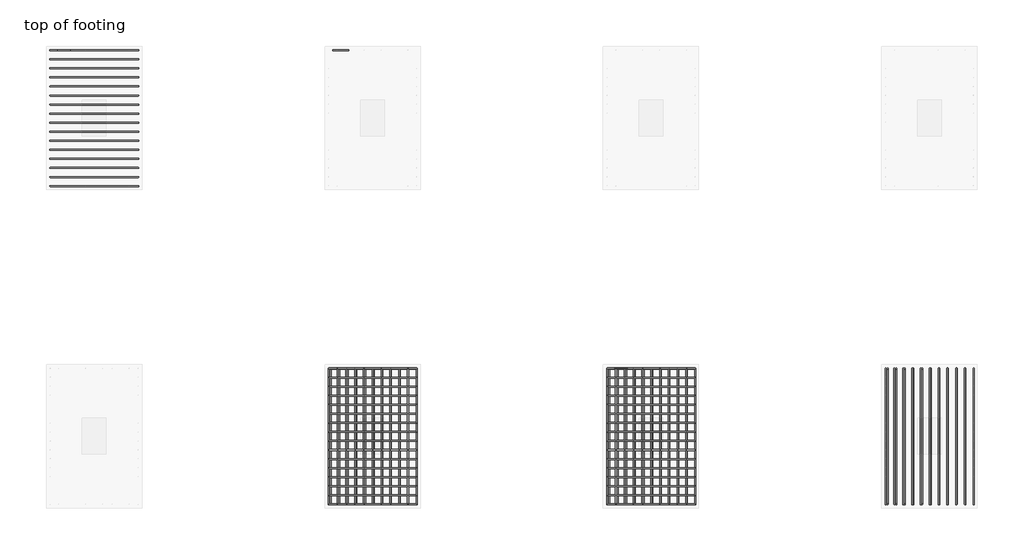
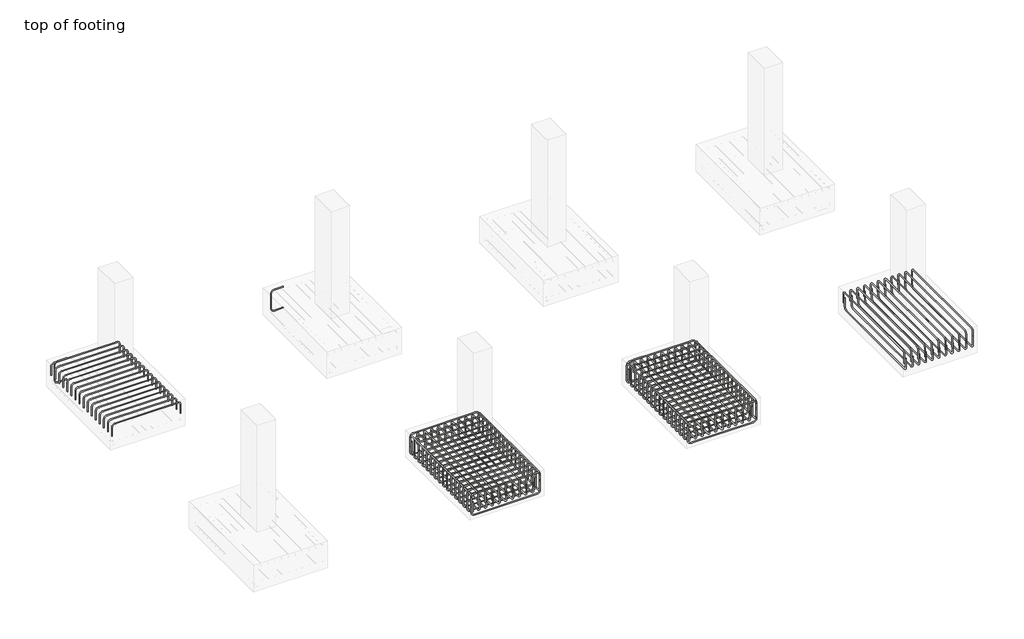
# One storey, part 4 of 8: 14 reinforcing bars.
"""IFC4 building model written with IfcOpenShell, lengths in millimetres."""

from ifc_helpers import new_model, si_unit, point, frame, origin, place, context, project, spatial, polyline, circle_curve, trimmed, segment, composite_curve, source, transform, mapped, element, save
from ifc_brep_helpers import swept_disk

model = new_model("IFC4")

# Units and contexts
model_context = context("Model", 3, world=origin())
ifc_project = project(units=[si_unit("LENGTHUNIT", "METRE", prefix="MILLI")], contexts=[model_context])

# Site, building, storey
site = spatial("IfcSite", under=ifc_project)
building = spatial("IfcBuilding", under=site)
storey = spatial("IfcBuildingStorey", under=building, Name="top of footing", Elevation=-1828.8)

# Reinforcing bars
placement = place(None, origin())
element("IfcReinforcingBar", 1, at=placement, inside=storey, context=model_context, shape_type="SolidModel", body=[
    swept_disk(composite_curve([segment(polyline([(-11543.0309105, 14390.1075251, -2232.45), (-11690.3309105, 14390.1075251, -2232.45)]), True, "CONTINUOUS"), segment(trimmed(circle_curve(frame((-11690.3309105, 14390.1075251, -2186.1), z_axis=(0.0, 1.0, 0.0), x_axis=(0.0, 0.0, -46.34999999999991)), 46.35), [point((-11690.3309105, 14390.1075251, -2232.45))], [point((-11736.6809105, 14390.1075251, -2186.1))], True, "CARTESIAN"), True, "CONTINUOUS"), segment(polyline([(-11736.6809105, 14390.1075251, -2186.1), (-11736.6809105, 14390.1075251, -1921.5)]), True, "CONTINUOUS"), segment(trimmed(circle_curve(frame((-11690.3309105, 14390.1075251, -1921.5), z_axis=(0.0, 1.0, 0.0), x_axis=(-46.349999999998545, 0.0, 0.0)), 46.35), [point((-11736.6809105, 14390.1075251, -1921.5))], [point((-11690.3309105, 14390.1075251, -1875.15))], True, "CARTESIAN"), True, "CONTINUOUS"), segment(polyline([(-11690.3309105, 14390.1075251, -1875.15), (-11543.0309105, 14390.1075251, -1875.15)]), True, "CONTINUOUS")], self_intersect=False), 6.35),
])
reinforcing_bar_shape = source(origin(), model_context, "Body", "SolidModel", [
    swept_disk(composite_curve([segment(polyline([(-11792.7300189, 14390.1075251, -2075.0801535), (-11792.7300189, 14390.1075251, -1927.7801535)]), True, "CONTINUOUS"), segment(trimmed(circle_curve(frame((-11746.3800189, 14390.1075251, -1927.7801535), z_axis=(0.0, 1.0, 0.0), x_axis=(-46.350000000000364, 0.0, 0.0)), 46.35), [point((-11792.7300189, 14390.1075251, -1927.7801535))], [point((-11746.3800189, 14390.1075251, -1881.4301535))], True, "CARTESIAN"), True, "CONTINUOUS"), segment(polyline([(-11746.3800189, 14390.1075251, -1881.4301535), (-10731.7800189, 14390.1075251, -1881.4301535)]), True, "CONTINUOUS"), segment(trimmed(circle_curve(frame((-10731.7800189, 14390.1075251, -1927.7801535), z_axis=(0.0, 1.0, 0.0), x_axis=(0.0, 0.0, 46.350000000000136)), 46.35), [point((-10731.7800189, 14390.1075251, -1881.4301535))], [point((-10685.4300189, 14390.1075251, -1927.7801535))], True, "CARTESIAN"), True, "CONTINUOUS"), segment(polyline([(-10685.4300189, 14390.1075251, -1927.7801535), (-10685.4300189, 14390.1075251, -2075.0801535)]), True, "CONTINUOUS")], self_intersect=False), 6.35),
])
element("IfcReinforcingBar", 2, at=placement, inside=storey, context=model_context, shape_type="MappedRepresentation", body=[
    mapped(reinforcing_bar_shape, transform((0.0, 0.0, 0.0), x_axis=(1.0, 0.0, 0.0), y_axis=(0.0, 1.0, 0.0), z_axis=(0.0, 0.0, 1.0))),
    mapped(reinforcing_bar_shape, transform((0.0, -113.82, 0.0), x_axis=(1.0, 0.0, 0.0), y_axis=(0.0, 1.0, 0.0), z_axis=(0.0, 0.0, 1.0))),
    mapped(reinforcing_bar_shape, transform((0.0, -227.64, 0.0), x_axis=(1.0, 0.0, 0.0), y_axis=(0.0, 1.0, 0.0), z_axis=(0.0, 0.0, 1.0))),
    mapped(reinforcing_bar_shape, transform((0.0, -341.46, 0.0), x_axis=(1.0, 0.0, 0.0), y_axis=(0.0, 1.0, 0.0), z_axis=(0.0, 0.0, 1.0))),
    mapped(reinforcing_bar_shape, transform((0.0, -455.28, 0.0), x_axis=(1.0, 0.0, 0.0), y_axis=(0.0, 1.0, 0.0), z_axis=(0.0, 0.0, 1.0))),
    mapped(reinforcing_bar_shape, transform((0.0, -569.1, 0.0), x_axis=(1.0, 0.0, 0.0), y_axis=(0.0, 1.0, 0.0), z_axis=(0.0, 0.0, 1.0))),
    mapped(reinforcing_bar_shape, transform((0.0, -682.92, 0.0), x_axis=(1.0, 0.0, 0.0), y_axis=(0.0, 1.0, 0.0), z_axis=(0.0, 0.0, 1.0))),
    mapped(reinforcing_bar_shape, transform((0.0, -796.74, 0.0), x_axis=(1.0, 0.0, 0.0), y_axis=(0.0, 1.0, 0.0), z_axis=(0.0, 0.0, 1.0))),
    mapped(reinforcing_bar_shape, transform((0.0, -910.56, 0.0), x_axis=(1.0, 0.0, 0.0), y_axis=(0.0, 1.0, 0.0), z_axis=(0.0, 0.0, 1.0))),
    mapped(reinforcing_bar_shape, transform((0.0, -1024.38, 0.0), x_axis=(1.0, 0.0, 0.0), y_axis=(0.0, 1.0, 0.0), z_axis=(0.0, 0.0, 1.0))),
    mapped(reinforcing_bar_shape, transform((0.0, -1138.2, 0.0), x_axis=(1.0, 0.0, 0.0), y_axis=(0.0, 1.0, 0.0), z_axis=(0.0, 0.0, 1.0))),
    mapped(reinforcing_bar_shape, transform((0.0, -1252.02, 0.0), x_axis=(1.0, 0.0, 0.0), y_axis=(0.0, 1.0, 0.0), z_axis=(0.0, 0.0, 1.0))),
    mapped(reinforcing_bar_shape, transform((0.0, -1365.84, 0.0), x_axis=(1.0, 0.0, 0.0), y_axis=(0.0, 1.0, 0.0), z_axis=(0.0, 0.0, 1.0))),
    mapped(reinforcing_bar_shape, transform((0.0, -1479.66, 0.0), x_axis=(1.0, 0.0, 0.0), y_axis=(0.0, 1.0, 0.0), z_axis=(0.0, 0.0, 1.0))),
    mapped(reinforcing_bar_shape, transform((0.0, -1593.48, 0.0), x_axis=(1.0, 0.0, 0.0), y_axis=(0.0, 1.0, 0.0), z_axis=(0.0, 0.0, 1.0))),
    mapped(reinforcing_bar_shape, transform((0.0, -1707.3, 0.0), x_axis=(1.0, 0.0, 0.0), y_axis=(0.0, 1.0, 0.0), z_axis=(0.0, 0.0, 1.0))),
])
element("IfcReinforcingBar", 3, at=placement, inside=storey, context=model_context, shape_type="SolidModel", body=[
    swept_disk(composite_curve([segment(polyline([(-8043.0309105, 14390.1075251, -2232.45), (-8190.3309105, 14390.1075251, -2232.45)]), True, "CONTINUOUS"), segment(trimmed(circle_curve(frame((-8190.3309105, 14390.1075251, -2186.1), z_axis=(0.0, 1.0, 0.0), x_axis=(0.0, 0.0, -46.34999999999991)), 46.35), [point((-8190.3309105, 14390.1075251, -2232.45))], [point((-8236.6809105, 14390.1075251, -2186.1))], True, "CARTESIAN"), True, "CONTINUOUS"), segment(polyline([(-8236.6809105, 14390.1075251, -2186.1), (-8236.6809105, 14390.1075251, -1921.5)]), True, "CONTINUOUS"), segment(trimmed(circle_curve(frame((-8190.3309105, 14390.1075251, -1921.5), z_axis=(0.0, 1.0, 0.0), x_axis=(-46.349999999999454, 0.0, 0.0)), 46.35), [point((-8236.6809105, 14390.1075251, -1921.5))], [point((-8190.3309105, 14390.1075251, -1875.15))], True, "CARTESIAN"), True, "CONTINUOUS"), segment(polyline([(-8190.3309105, 14390.1075251, -1875.15), (-8043.0309105, 14390.1075251, -1875.15)]), True, "CONTINUOUS")], self_intersect=False), 6.35),
])
reinforcing_bar_2_shape = source(origin(), model_context, "Body", "SolidModel", [
    swept_disk(composite_curve([segment(polyline([(-185.4300189, 8682.8075251, -2014.4920065), (-185.4300189, 8682.8075251, -2161.7920065)]), True, "CONTINUOUS"), segment(trimmed(circle_curve(frame((-185.4300189, 8729.1575251, -2161.7920065), z_axis=(1.0, 0.0, 0.0), x_axis=(0.0, -46.350000000000364, 0.0)), 46.35), [point((-185.4300189, 8682.8075251, -2161.7920065))], [point((-185.4300189, 8729.1575251, -2208.1420065))], True, "CARTESIAN"), True, "CONTINUOUS"), segment(polyline([(-185.4300189, 8729.1575251, -2208.1420065), (-185.4300189, 10343.7575251, -2208.1420065)]), True, "CONTINUOUS"), segment(trimmed(circle_curve(frame((-185.4300189, 10343.7575251, -2161.7920065), z_axis=(1.0, 0.0, 0.0), x_axis=(0.0, 0.0, -46.350000000000364)), 46.35), [point((-185.4300189, 10343.7575251, -2208.1420065))], [point((-185.4300189, 10390.1075251, -2161.7920065))], True, "CARTESIAN"), True, "CONTINUOUS"), segment(polyline([(-185.4300189, 10390.1075251, -2161.7920065), (-185.4300189, 10390.1075251, -2014.4920065)]), True, "CONTINUOUS")], self_intersect=False), 6.35),
])
element("IfcReinforcingBar", 4, at=placement, inside=storey, context=model_context, shape_type="MappedRepresentation", body=[
    mapped(reinforcing_bar_2_shape, transform((0.0, 0.0, 0.0), x_axis=(1.0, 0.0, 0.0), y_axis=(0.0, 1.0, 0.0), z_axis=(0.0, 0.0, 1.0))),
    mapped(reinforcing_bar_2_shape, transform((-108.3645139, 0.0, 0.0), x_axis=(1.0, 0.0, 0.0), y_axis=(0.0, 1.0, 0.0), z_axis=(0.0, 0.0, 1.0))),
    mapped(reinforcing_bar_2_shape, transform((-216.7290279, 0.0, 0.0), x_axis=(1.0, 0.0, 0.0), y_axis=(0.0, 1.0, 0.0), z_axis=(0.0, 0.0, 1.0))),
    mapped(reinforcing_bar_2_shape, transform((-325.0935418, 0.0, 0.0), x_axis=(1.0, 0.0, 0.0), y_axis=(0.0, 1.0, 0.0), z_axis=(0.0, 0.0, 1.0))),
    mapped(reinforcing_bar_2_shape, transform((-433.4580557, 0.0, 0.0), x_axis=(1.0, 0.0, 0.0), y_axis=(0.0, 1.0, 0.0), z_axis=(0.0, 0.0, 1.0))),
    mapped(reinforcing_bar_2_shape, transform((-541.8225696, 0.0, 0.0), x_axis=(1.0, 0.0, 0.0), y_axis=(0.0, 1.0, 0.0), z_axis=(0.0, 0.0, 1.0))),
    mapped(reinforcing_bar_2_shape, transform((-650.1870836, 0.0, 0.0), x_axis=(1.0, 0.0, 0.0), y_axis=(0.0, 1.0, 0.0), z_axis=(0.0, 0.0, 1.0))),
    mapped(reinforcing_bar_2_shape, transform((-758.5515975, 0.0, 0.0), x_axis=(1.0, 0.0, 0.0), y_axis=(0.0, 1.0, 0.0), z_axis=(0.0, 0.0, 1.0))),
    mapped(reinforcing_bar_2_shape, transform((-866.9161114, 0.0, 0.0), x_axis=(1.0, 0.0, 0.0), y_axis=(0.0, 1.0, 0.0), z_axis=(0.0, 0.0, 1.0))),
    mapped(reinforcing_bar_2_shape, transform((-975.2806253, 0.0, 0.0), x_axis=(1.0, 0.0, 0.0), y_axis=(0.0, 1.0, 0.0), z_axis=(0.0, 0.0, 1.0))),
    mapped(reinforcing_bar_2_shape, transform((-1083.6451393, 0.0, 0.0), x_axis=(1.0, 0.0, 0.0), y_axis=(0.0, 1.0, 0.0), z_axis=(0.0, 0.0, 1.0))),
])
reinforcing_bar_3_shape = source(origin(), model_context, "Body", "SolidModel", [
    swept_disk(composite_curve([segment(polyline([(-1292.7300189, 8682.8075251, -2085.8010212), (-1292.7300189, 8682.8075251, -1938.5010212)]), True, "CONTINUOUS"), segment(trimmed(circle_curve(frame((-1292.7300189, 8729.1575251, -1938.5010212), z_axis=(-1.0, 0.0, 0.0), x_axis=(0.0, -46.350000000000364, 0.0)), 46.35), [point((-1292.7300189, 8682.8075251, -1938.5010212))], [point((-1292.7300189, 8729.1575251, -1892.1510212))], True, "CARTESIAN"), True, "CONTINUOUS"), segment(polyline([(-1292.7300189, 8729.1575251, -1892.1510212), (-1292.7300189, 10343.7575251, -1892.1510212)]), True, "CONTINUOUS"), segment(trimmed(circle_curve(frame((-1292.7300189, 10343.7575251, -1938.5010212), z_axis=(-1.0, 0.0, 0.0), x_axis=(0.0, 0.0, 46.34999999999991)), 46.35), [point((-1292.7300189, 10343.7575251, -1892.1510212))], [point((-1292.7300189, 10390.1075251, -1938.5010212))], True, "CARTESIAN"), True, "CONTINUOUS"), segment(polyline([(-1292.7300189, 10390.1075251, -1938.5010212), (-1292.7300189, 10390.1075251, -2085.8010212)]), True, "CONTINUOUS")], self_intersect=False), 6.35),
])
element("IfcReinforcingBar", 5, at=placement, inside=storey, context=model_context, shape_type="MappedRepresentation", body=[
    mapped(reinforcing_bar_3_shape, transform((0.0, 0.0, 0.0), x_axis=(1.0, 0.0, 0.0), y_axis=(0.0, 1.0, 0.0), z_axis=(0.0, 0.0, 1.0))),
    mapped(reinforcing_bar_3_shape, transform((110.73, 0.0, 0.0), x_axis=(1.0, 0.0, 0.0), y_axis=(0.0, 1.0, 0.0), z_axis=(0.0, 0.0, 1.0))),
    mapped(reinforcing_bar_3_shape, transform((221.46, 0.0, 0.0), x_axis=(1.0, 0.0, 0.0), y_axis=(0.0, 1.0, 0.0), z_axis=(0.0, 0.0, 1.0))),
    mapped(reinforcing_bar_3_shape, transform((332.19, 0.0, 0.0), x_axis=(1.0, 0.0, 0.0), y_axis=(0.0, 1.0, 0.0), z_axis=(0.0, 0.0, 1.0))),
    mapped(reinforcing_bar_3_shape, transform((442.92, 0.0, 0.0), x_axis=(1.0, 0.0, 0.0), y_axis=(0.0, 1.0, 0.0), z_axis=(0.0, 0.0, 1.0))),
    mapped(reinforcing_bar_3_shape, transform((553.65, 0.0, 0.0), x_axis=(1.0, 0.0, 0.0), y_axis=(0.0, 1.0, 0.0), z_axis=(0.0, 0.0, 1.0))),
    mapped(reinforcing_bar_3_shape, transform((664.38, 0.0, 0.0), x_axis=(1.0, 0.0, 0.0), y_axis=(0.0, 1.0, 0.0), z_axis=(0.0, 0.0, 1.0))),
    mapped(reinforcing_bar_3_shape, transform((775.11, 0.0, 0.0), x_axis=(1.0, 0.0, 0.0), y_axis=(0.0, 1.0, 0.0), z_axis=(0.0, 0.0, 1.0))),
    mapped(reinforcing_bar_3_shape, transform((885.84, 0.0, 0.0), x_axis=(1.0, 0.0, 0.0), y_axis=(0.0, 1.0, 0.0), z_axis=(0.0, 0.0, 1.0))),
    mapped(reinforcing_bar_3_shape, transform((996.57, 0.0, 0.0), x_axis=(1.0, 0.0, 0.0), y_axis=(0.0, 1.0, 0.0), z_axis=(0.0, 0.0, 1.0))),
    mapped(reinforcing_bar_3_shape, transform((1107.3, 0.0, 0.0), x_axis=(1.0, 0.0, 0.0), y_axis=(0.0, 1.0, 0.0), z_axis=(0.0, 0.0, 1.0))),
])
reinforcing_bar_4_shape = source(origin(), model_context, "Body", "SolidModel", [
    swept_disk(composite_curve([segment(polyline([(-3685.4300189, 8682.8075251, -2014.4920065), (-3685.4300189, 8682.8075251, -2161.7920065)]), True, "CONTINUOUS"), segment(trimmed(circle_curve(frame((-3685.4300189, 8729.1575251, -2161.7920065), z_axis=(1.0, 0.0, 0.0), x_axis=(0.0, -46.350000000000364, 0.0)), 46.35), [point((-3685.4300189, 8682.8075251, -2161.7920065))], [point((-3685.4300189, 8729.1575251, -2208.1420065))], True, "CARTESIAN"), True, "CONTINUOUS"), segment(polyline([(-3685.4300189, 8729.1575251, -2208.1420065), (-3685.4300189, 10343.7575251, -2208.1420065)]), True, "CONTINUOUS"), segment(trimmed(circle_curve(frame((-3685.4300189, 10343.7575251, -2161.7920065), z_axis=(1.0, 0.0, 0.0), x_axis=(0.0, 0.0, -46.350000000000364)), 46.35), [point((-3685.4300189, 10343.7575251, -2208.1420065))], [point((-3685.4300189, 10390.1075251, -2161.7920065))], True, "CARTESIAN"), True, "CONTINUOUS"), segment(polyline([(-3685.4300189, 10390.1075251, -2161.7920065), (-3685.4300189, 10390.1075251, -2014.4920065)]), True, "CONTINUOUS")], self_intersect=False), 6.35),
])
element("IfcReinforcingBar", 6, at=placement, inside=storey, context=model_context, shape_type="MappedRepresentation", body=[
    mapped(reinforcing_bar_4_shape, transform((0.0, 0.0, 0.0), x_axis=(1.0, 0.0, 0.0), y_axis=(0.0, 1.0, 0.0), z_axis=(0.0, 0.0, 1.0))),
    mapped(reinforcing_bar_4_shape, transform((-108.3645139, 0.0, 0.0), x_axis=(1.0, 0.0, 0.0), y_axis=(0.0, 1.0, 0.0), z_axis=(0.0, 0.0, 1.0))),
    mapped(reinforcing_bar_4_shape, transform((-216.7290279, 0.0, 0.0), x_axis=(1.0, 0.0, 0.0), y_axis=(0.0, 1.0, 0.0), z_axis=(0.0, 0.0, 1.0))),
    mapped(reinforcing_bar_4_shape, transform((-325.0935418, 0.0, 0.0), x_axis=(1.0, 0.0, 0.0), y_axis=(0.0, 1.0, 0.0), z_axis=(0.0, 0.0, 1.0))),
    mapped(reinforcing_bar_4_shape, transform((-433.4580557, 0.0, 0.0), x_axis=(1.0, 0.0, 0.0), y_axis=(0.0, 1.0, 0.0), z_axis=(0.0, 0.0, 1.0))),
    mapped(reinforcing_bar_4_shape, transform((-541.8225696, 0.0, 0.0), x_axis=(1.0, 0.0, 0.0), y_axis=(0.0, 1.0, 0.0), z_axis=(0.0, 0.0, 1.0))),
    mapped(reinforcing_bar_4_shape, transform((-650.1870836, 0.0, 0.0), x_axis=(1.0, 0.0, 0.0), y_axis=(0.0, 1.0, 0.0), z_axis=(0.0, 0.0, 1.0))),
    mapped(reinforcing_bar_4_shape, transform((-758.5515975, 0.0, 0.0), x_axis=(1.0, 0.0, 0.0), y_axis=(0.0, 1.0, 0.0), z_axis=(0.0, 0.0, 1.0))),
    mapped(reinforcing_bar_4_shape, transform((-866.9161114, 0.0, 0.0), x_axis=(1.0, 0.0, 0.0), y_axis=(0.0, 1.0, 0.0), z_axis=(0.0, 0.0, 1.0))),
    mapped(reinforcing_bar_4_shape, transform((-975.2806253, 0.0, 0.0), x_axis=(1.0, 0.0, 0.0), y_axis=(0.0, 1.0, 0.0), z_axis=(0.0, 0.0, 1.0))),
    mapped(reinforcing_bar_4_shape, transform((-1083.6451393, 0.0, 0.0), x_axis=(1.0, 0.0, 0.0), y_axis=(0.0, 1.0, 0.0), z_axis=(0.0, 0.0, 1.0))),
])
reinforcing_bar_5_shape = source(origin(), model_context, "Body", "SolidModel", [
    swept_disk(composite_curve([segment(polyline([(-4792.7300189, 8682.8075251, -2085.8010212), (-4792.7300189, 8682.8075251, -1938.5010212)]), True, "CONTINUOUS"), segment(trimmed(circle_curve(frame((-4792.7300189, 8729.1575251, -1938.5010212), z_axis=(-1.0, 0.0, 0.0), x_axis=(0.0, -46.350000000000364, 0.0)), 46.35), [point((-4792.7300189, 8682.8075251, -1938.5010212))], [point((-4792.7300189, 8729.1575251, -1892.1510212))], True, "CARTESIAN"), True, "CONTINUOUS"), segment(polyline([(-4792.7300189, 8729.1575251, -1892.1510212), (-4792.7300189, 10343.7575251, -1892.1510212)]), True, "CONTINUOUS"), segment(trimmed(circle_curve(frame((-4792.7300189, 10343.7575251, -1938.5010212), z_axis=(-1.0, 0.0, 0.0), x_axis=(0.0, 0.0, 46.34999999999991)), 46.35), [point((-4792.7300189, 10343.7575251, -1892.1510212))], [point((-4792.7300189, 10390.1075251, -1938.5010212))], True, "CARTESIAN"), True, "CONTINUOUS"), segment(polyline([(-4792.7300189, 10390.1075251, -1938.5010212), (-4792.7300189, 10390.1075251, -2085.8010212)]), True, "CONTINUOUS")], self_intersect=False), 6.35),
])
element("IfcReinforcingBar", 7, at=placement, inside=storey, context=model_context, shape_type="MappedRepresentation", body=[
    mapped(reinforcing_bar_5_shape, transform((0.0, 0.0, 0.0), x_axis=(1.0, 0.0, 0.0), y_axis=(0.0, 1.0, 0.0), z_axis=(0.0, 0.0, 1.0))),
    mapped(reinforcing_bar_5_shape, transform((110.73, 0.0, 0.0), x_axis=(1.0, 0.0, 0.0), y_axis=(0.0, 1.0, 0.0), z_axis=(0.0, 0.0, 1.0))),
    mapped(reinforcing_bar_5_shape, transform((221.46, 0.0, 0.0), x_axis=(1.0, 0.0, 0.0), y_axis=(0.0, 1.0, 0.0), z_axis=(0.0, 0.0, 1.0))),
    mapped(reinforcing_bar_5_shape, transform((332.19, 0.0, 0.0), x_axis=(1.0, 0.0, 0.0), y_axis=(0.0, 1.0, 0.0), z_axis=(0.0, 0.0, 1.0))),
    mapped(reinforcing_bar_5_shape, transform((442.92, 0.0, 0.0), x_axis=(1.0, 0.0, 0.0), y_axis=(0.0, 1.0, 0.0), z_axis=(0.0, 0.0, 1.0))),
    mapped(reinforcing_bar_5_shape, transform((553.65, 0.0, 0.0), x_axis=(1.0, 0.0, 0.0), y_axis=(0.0, 1.0, 0.0), z_axis=(0.0, 0.0, 1.0))),
    mapped(reinforcing_bar_5_shape, transform((664.38, 0.0, 0.0), x_axis=(1.0, 0.0, 0.0), y_axis=(0.0, 1.0, 0.0), z_axis=(0.0, 0.0, 1.0))),
    mapped(reinforcing_bar_5_shape, transform((775.11, 0.0, 0.0), x_axis=(1.0, 0.0, 0.0), y_axis=(0.0, 1.0, 0.0), z_axis=(0.0, 0.0, 1.0))),
    mapped(reinforcing_bar_5_shape, transform((885.84, 0.0, 0.0), x_axis=(1.0, 0.0, 0.0), y_axis=(0.0, 1.0, 0.0), z_axis=(0.0, 0.0, 1.0))),
    mapped(reinforcing_bar_5_shape, transform((996.57, 0.0, 0.0), x_axis=(1.0, 0.0, 0.0), y_axis=(0.0, 1.0, 0.0), z_axis=(0.0, 0.0, 1.0))),
    mapped(reinforcing_bar_5_shape, transform((1107.3, 0.0, 0.0), x_axis=(1.0, 0.0, 0.0), y_axis=(0.0, 1.0, 0.0), z_axis=(0.0, 0.0, 1.0))),
])
element("IfcReinforcingBar", 8, at=placement, inside=storey, context=model_context, shape_type="SolidModel", body=[
    swept_disk(composite_curve([segment(polyline([(-4543.0309105, 10390.1075251, -2232.45), (-4690.3309105, 10390.1075251, -2232.45)]), True, "CONTINUOUS"), segment(trimmed(circle_curve(frame((-4690.3309105, 10390.1075251, -2186.1), z_axis=(0.0, 1.0, 0.0), x_axis=(0.0, 0.0, -46.34999999999991)), 46.35), [point((-4690.3309105, 10390.1075251, -2232.45))], [point((-4736.6809105, 10390.1075251, -2186.1))], True, "CARTESIAN"), True, "CONTINUOUS"), segment(polyline([(-4736.6809105, 10390.1075251, -2186.1), (-4736.6809105, 10390.1075251, -1921.5)]), True, "CONTINUOUS"), segment(trimmed(circle_curve(frame((-4690.3309105, 10390.1075251, -1921.5), z_axis=(0.0, 1.0, 0.0), x_axis=(-46.350000000000364, 0.0, 0.0)), 46.35), [point((-4736.6809105, 10390.1075251, -1921.5))], [point((-4690.3309105, 10390.1075251, -1875.15))], True, "CARTESIAN"), True, "CONTINUOUS"), segment(polyline([(-4690.3309105, 10390.1075251, -1875.15), (-4543.0309105, 10390.1075251, -1875.15)]), True, "CONTINUOUS")], self_intersect=False), 6.35),
])
reinforcing_bar_6_shape = source(origin(), model_context, "Body", "SolidModel", [
    swept_disk(composite_curve([segment(polyline([(-3685.4300189, 10390.1075251, -2044.8290141), (-3685.4300189, 10390.1075251, -2192.1290141)]), True, "CONTINUOUS"), segment(trimmed(circle_curve(frame((-3731.7800189, 10390.1075251, -2192.1290141), z_axis=(0.0, 1.0, 0.0), x_axis=(46.34999999999991, 0.0, 0.0)), 46.35), [point((-3685.4300189, 10390.1075251, -2192.1290141))], [point((-3731.7800189, 10390.1075251, -2238.4790141))], True, "CARTESIAN"), True, "CONTINUOUS"), segment(polyline([(-3731.7800189, 10390.1075251, -2238.4790141), (-4746.3800189, 10390.1075251, -2238.4790141)]), True, "CONTINUOUS"), segment(trimmed(circle_curve(frame((-4746.3800189, 10390.1075251, -2192.1290141), z_axis=(0.0, 1.0, 0.0), x_axis=(0.0, 0.0, -46.34999999999991)), 46.35), [point((-4746.3800189, 10390.1075251, -2238.4790141))], [point((-4792.7300189, 10390.1075251, -2192.1290141))], True, "CARTESIAN"), True, "CONTINUOUS"), segment(polyline([(-4792.7300189, 10390.1075251, -2192.1290141), (-4792.7300189, 10390.1075251, -2044.8290141)]), True, "CONTINUOUS")], self_intersect=False), 6.35),
])
element("IfcReinforcingBar", 9, at=placement, inside=storey, context=model_context, shape_type="MappedRepresentation", body=[
    mapped(reinforcing_bar_6_shape, transform((0.0, 0.0, 0.0), x_axis=(1.0, 0.0, 0.0), y_axis=(0.0, 1.0, 0.0), z_axis=(0.0, 0.0, 1.0))),
    mapped(reinforcing_bar_6_shape, transform((0.0, -113.82, 0.0), x_axis=(1.0, 0.0, 0.0), y_axis=(0.0, 1.0, 0.0), z_axis=(0.0, 0.0, 1.0))),
    mapped(reinforcing_bar_6_shape, transform((0.0, -227.64, 0.0), x_axis=(1.0, 0.0, 0.0), y_axis=(0.0, 1.0, 0.0), z_axis=(0.0, 0.0, 1.0))),
    mapped(reinforcing_bar_6_shape, transform((0.0, -341.46, 0.0), x_axis=(1.0, 0.0, 0.0), y_axis=(0.0, 1.0, 0.0), z_axis=(0.0, 0.0, 1.0))),
    mapped(reinforcing_bar_6_shape, transform((0.0, -455.28, 0.0), x_axis=(1.0, 0.0, 0.0), y_axis=(0.0, 1.0, 0.0), z_axis=(0.0, 0.0, 1.0))),
    mapped(reinforcing_bar_6_shape, transform((0.0, -569.1, 0.0), x_axis=(1.0, 0.0, 0.0), y_axis=(0.0, 1.0, 0.0), z_axis=(0.0, 0.0, 1.0))),
    mapped(reinforcing_bar_6_shape, transform((0.0, -682.92, 0.0), x_axis=(1.0, 0.0, 0.0), y_axis=(0.0, 1.0, 0.0), z_axis=(0.0, 0.0, 1.0))),
    mapped(reinforcing_bar_6_shape, transform((0.0, -796.74, 0.0), x_axis=(1.0, 0.0, 0.0), y_axis=(0.0, 1.0, 0.0), z_axis=(0.0, 0.0, 1.0))),
    mapped(reinforcing_bar_6_shape, transform((0.0, -910.56, 0.0), x_axis=(1.0, 0.0, 0.0), y_axis=(0.0, 1.0, 0.0), z_axis=(0.0, 0.0, 1.0))),
    mapped(reinforcing_bar_6_shape, transform((0.0, -1024.38, 0.0), x_axis=(1.0, 0.0, 0.0), y_axis=(0.0, 1.0, 0.0), z_axis=(0.0, 0.0, 1.0))),
    mapped(reinforcing_bar_6_shape, transform((0.0, -1138.2, 0.0), x_axis=(1.0, 0.0, 0.0), y_axis=(0.0, 1.0, 0.0), z_axis=(0.0, 0.0, 1.0))),
    mapped(reinforcing_bar_6_shape, transform((0.0, -1252.02, 0.0), x_axis=(1.0, 0.0, 0.0), y_axis=(0.0, 1.0, 0.0), z_axis=(0.0, 0.0, 1.0))),
    mapped(reinforcing_bar_6_shape, transform((0.0, -1365.84, 0.0), x_axis=(1.0, 0.0, 0.0), y_axis=(0.0, 1.0, 0.0), z_axis=(0.0, 0.0, 1.0))),
    mapped(reinforcing_bar_6_shape, transform((0.0, -1479.66, 0.0), x_axis=(1.0, 0.0, 0.0), y_axis=(0.0, 1.0, 0.0), z_axis=(0.0, 0.0, 1.0))),
    mapped(reinforcing_bar_6_shape, transform((0.0, -1593.48, 0.0), x_axis=(1.0, 0.0, 0.0), y_axis=(0.0, 1.0, 0.0), z_axis=(0.0, 0.0, 1.0))),
    mapped(reinforcing_bar_6_shape, transform((0.0, -1707.3, 0.0), x_axis=(1.0, 0.0, 0.0), y_axis=(0.0, 1.0, 0.0), z_axis=(0.0, 0.0, 1.0))),
])
reinforcing_bar_7_shape = source(origin(), model_context, "Body", "SolidModel", [
    swept_disk(composite_curve([segment(polyline([(-4792.7300189, 10390.1075251, -2075.0801535), (-4792.7300189, 10390.1075251, -1927.7801535)]), True, "CONTINUOUS"), segment(trimmed(circle_curve(frame((-4746.3800189, 10390.1075251, -1927.7801535), z_axis=(0.0, 1.0, 0.0), x_axis=(-46.349999999999454, 0.0, 0.0)), 46.35), [point((-4792.7300189, 10390.1075251, -1927.7801535))], [point((-4746.3800189, 10390.1075251, -1881.4301535))], True, "CARTESIAN"), True, "CONTINUOUS"), segment(polyline([(-4746.3800189, 10390.1075251, -1881.4301535), (-3731.7800189, 10390.1075251, -1881.4301535)]), True, "CONTINUOUS"), segment(trimmed(circle_curve(frame((-3731.7800189, 10390.1075251, -1927.7801535), z_axis=(0.0, 1.0, 0.0), x_axis=(0.0, 0.0, 46.350000000000136)), 46.35), [point((-3731.7800189, 10390.1075251, -1881.4301535))], [point((-3685.4300189, 10390.1075251, -1927.7801535))], True, "CARTESIAN"), True, "CONTINUOUS"), segment(polyline([(-3685.4300189, 10390.1075251, -1927.7801535), (-3685.4300189, 10390.1075251, -2075.0801535)]), True, "CONTINUOUS")], self_intersect=False), 6.35),
])
element("IfcReinforcingBar", 10, at=placement, inside=storey, context=model_context, shape_type="MappedRepresentation", body=[
    mapped(reinforcing_bar_7_shape, transform((0.0, 0.0, 0.0), x_axis=(1.0, 0.0, 0.0), y_axis=(0.0, 1.0, 0.0), z_axis=(0.0, 0.0, 1.0))),
    mapped(reinforcing_bar_7_shape, transform((0.0, -113.82, 0.0), x_axis=(1.0, 0.0, 0.0), y_axis=(0.0, 1.0, 0.0), z_axis=(0.0, 0.0, 1.0))),
    mapped(reinforcing_bar_7_shape, transform((0.0, -227.64, 0.0), x_axis=(1.0, 0.0, 0.0), y_axis=(0.0, 1.0, 0.0), z_axis=(0.0, 0.0, 1.0))),
    mapped(reinforcing_bar_7_shape, transform((0.0, -341.46, 0.0), x_axis=(1.0, 0.0, 0.0), y_axis=(0.0, 1.0, 0.0), z_axis=(0.0, 0.0, 1.0))),
    mapped(reinforcing_bar_7_shape, transform((0.0, -455.28, 0.0), x_axis=(1.0, 0.0, 0.0), y_axis=(0.0, 1.0, 0.0), z_axis=(0.0, 0.0, 1.0))),
    mapped(reinforcing_bar_7_shape, transform((0.0, -569.1, 0.0), x_axis=(1.0, 0.0, 0.0), y_axis=(0.0, 1.0, 0.0), z_axis=(0.0, 0.0, 1.0))),
    mapped(reinforcing_bar_7_shape, transform((0.0, -682.92, 0.0), x_axis=(1.0, 0.0, 0.0), y_axis=(0.0, 1.0, 0.0), z_axis=(0.0, 0.0, 1.0))),
    mapped(reinforcing_bar_7_shape, transform((0.0, -796.74, 0.0), x_axis=(1.0, 0.0, 0.0), y_axis=(0.0, 1.0, 0.0), z_axis=(0.0, 0.0, 1.0))),
    mapped(reinforcing_bar_7_shape, transform((0.0, -910.56, 0.0), x_axis=(1.0, 0.0, 0.0), y_axis=(0.0, 1.0, 0.0), z_axis=(0.0, 0.0, 1.0))),
    mapped(reinforcing_bar_7_shape, transform((0.0, -1024.38, 0.0), x_axis=(1.0, 0.0, 0.0), y_axis=(0.0, 1.0, 0.0), z_axis=(0.0, 0.0, 1.0))),
    mapped(reinforcing_bar_7_shape, transform((0.0, -1138.2, 0.0), x_axis=(1.0, 0.0, 0.0), y_axis=(0.0, 1.0, 0.0), z_axis=(0.0, 0.0, 1.0))),
    mapped(reinforcing_bar_7_shape, transform((0.0, -1252.02, 0.0), x_axis=(1.0, 0.0, 0.0), y_axis=(0.0, 1.0, 0.0), z_axis=(0.0, 0.0, 1.0))),
    mapped(reinforcing_bar_7_shape, transform((0.0, -1365.84, 0.0), x_axis=(1.0, 0.0, 0.0), y_axis=(0.0, 1.0, 0.0), z_axis=(0.0, 0.0, 1.0))),
    mapped(reinforcing_bar_7_shape, transform((0.0, -1479.66, 0.0), x_axis=(1.0, 0.0, 0.0), y_axis=(0.0, 1.0, 0.0), z_axis=(0.0, 0.0, 1.0))),
    mapped(reinforcing_bar_7_shape, transform((0.0, -1593.48, 0.0), x_axis=(1.0, 0.0, 0.0), y_axis=(0.0, 1.0, 0.0), z_axis=(0.0, 0.0, 1.0))),
    mapped(reinforcing_bar_7_shape, transform((0.0, -1707.3, 0.0), x_axis=(1.0, 0.0, 0.0), y_axis=(0.0, 1.0, 0.0), z_axis=(0.0, 0.0, 1.0))),
])
reinforcing_bar_8_shape = source(origin(), model_context, "Body", "SolidModel", [
    swept_disk(composite_curve([segment(polyline([(-7185.4300189, 8682.8075251, -2014.4920065), (-7185.4300189, 8682.8075251, -2161.7920065)]), True, "CONTINUOUS"), segment(trimmed(circle_curve(frame((-7185.4300189, 8729.1575251, -2161.7920065), z_axis=(1.0, 0.0, 0.0), x_axis=(0.0, -46.350000000000364, 0.0)), 46.35), [point((-7185.4300189, 8682.8075251, -2161.7920065))], [point((-7185.4300189, 8729.1575251, -2208.1420065))], True, "CARTESIAN"), True, "CONTINUOUS"), segment(polyline([(-7185.4300189, 8729.1575251, -2208.1420065), (-7185.4300189, 10343.7575251, -2208.1420065)]), True, "CONTINUOUS"), segment(trimmed(circle_curve(frame((-7185.4300189, 10343.7575251, -2161.7920065), z_axis=(1.0, 0.0, 0.0), x_axis=(0.0, 0.0, -46.350000000000364)), 46.35), [point((-7185.4300189, 10343.7575251, -2208.1420065))], [point((-7185.4300189, 10390.1075251, -2161.7920065))], True, "CARTESIAN"), True, "CONTINUOUS"), segment(polyline([(-7185.4300189, 10390.1075251, -2161.7920065), (-7185.4300189, 10390.1075251, -2014.4920065)]), True, "CONTINUOUS")], self_intersect=False), 6.35),
])
element("IfcReinforcingBar", 11, at=placement, inside=storey, context=model_context, shape_type="MappedRepresentation", body=[
    mapped(reinforcing_bar_8_shape, transform((0.0, 0.0, 0.0), x_axis=(1.0, 0.0, 0.0), y_axis=(0.0, 1.0, 0.0), z_axis=(0.0, 0.0, 1.0))),
    mapped(reinforcing_bar_8_shape, transform((-108.3645139, 0.0, 0.0), x_axis=(1.0, 0.0, 0.0), y_axis=(0.0, 1.0, 0.0), z_axis=(0.0, 0.0, 1.0))),
    mapped(reinforcing_bar_8_shape, transform((-216.7290279, 0.0, 0.0), x_axis=(1.0, 0.0, 0.0), y_axis=(0.0, 1.0, 0.0), z_axis=(0.0, 0.0, 1.0))),
    mapped(reinforcing_bar_8_shape, transform((-325.0935418, 0.0, 0.0), x_axis=(1.0, 0.0, 0.0), y_axis=(0.0, 1.0, 0.0), z_axis=(0.0, 0.0, 1.0))),
    mapped(reinforcing_bar_8_shape, transform((-433.4580557, 0.0, 0.0), x_axis=(1.0, 0.0, 0.0), y_axis=(0.0, 1.0, 0.0), z_axis=(0.0, 0.0, 1.0))),
    mapped(reinforcing_bar_8_shape, transform((-541.8225696, 0.0, 0.0), x_axis=(1.0, 0.0, 0.0), y_axis=(0.0, 1.0, 0.0), z_axis=(0.0, 0.0, 1.0))),
    mapped(reinforcing_bar_8_shape, transform((-650.1870836, 0.0, 0.0), x_axis=(1.0, 0.0, 0.0), y_axis=(0.0, 1.0, 0.0), z_axis=(0.0, 0.0, 1.0))),
    mapped(reinforcing_bar_8_shape, transform((-758.5515975, 0.0, 0.0), x_axis=(1.0, 0.0, 0.0), y_axis=(0.0, 1.0, 0.0), z_axis=(0.0, 0.0, 1.0))),
    mapped(reinforcing_bar_8_shape, transform((-866.9161114, 0.0, 0.0), x_axis=(1.0, 0.0, 0.0), y_axis=(0.0, 1.0, 0.0), z_axis=(0.0, 0.0, 1.0))),
    mapped(reinforcing_bar_8_shape, transform((-975.2806253, 0.0, 0.0), x_axis=(1.0, 0.0, 0.0), y_axis=(0.0, 1.0, 0.0), z_axis=(0.0, 0.0, 1.0))),
    mapped(reinforcing_bar_8_shape, transform((-1083.6451393, 0.0, 0.0), x_axis=(1.0, 0.0, 0.0), y_axis=(0.0, 1.0, 0.0), z_axis=(0.0, 0.0, 1.0))),
])
reinforcing_bar_9_shape = source(origin(), model_context, "Body", "SolidModel", [
    swept_disk(composite_curve([segment(polyline([(-8292.7300189, 8682.8075251, -2085.8010212), (-8292.7300189, 8682.8075251, -1938.5010212)]), True, "CONTINUOUS"), segment(trimmed(circle_curve(frame((-8292.7300189, 8729.1575251, -1938.5010212), z_axis=(-1.0, 0.0, 0.0), x_axis=(0.0, -46.350000000000364, 0.0)), 46.35), [point((-8292.7300189, 8682.8075251, -1938.5010212))], [point((-8292.7300189, 8729.1575251, -1892.1510212))], True, "CARTESIAN"), True, "CONTINUOUS"), segment(polyline([(-8292.7300189, 8729.1575251, -1892.1510212), (-8292.7300189, 10343.7575251, -1892.1510212)]), True, "CONTINUOUS"), segment(trimmed(circle_curve(frame((-8292.7300189, 10343.7575251, -1938.5010212), z_axis=(-1.0, 0.0, 0.0), x_axis=(0.0, 0.0, 46.34999999999991)), 46.35), [point((-8292.7300189, 10343.7575251, -1892.1510212))], [point((-8292.7300189, 10390.1075251, -1938.5010212))], True, "CARTESIAN"), True, "CONTINUOUS"), segment(polyline([(-8292.7300189, 10390.1075251, -1938.5010212), (-8292.7300189, 10390.1075251, -2085.8010212)]), True, "CONTINUOUS")], self_intersect=False), 6.35),
])
element("IfcReinforcingBar", 12, at=placement, inside=storey, context=model_context, shape_type="MappedRepresentation", body=[
    mapped(reinforcing_bar_9_shape, transform((0.0, 0.0, 0.0), x_axis=(1.0, 0.0, 0.0), y_axis=(0.0, 1.0, 0.0), z_axis=(0.0, 0.0, 1.0))),
    mapped(reinforcing_bar_9_shape, transform((110.73, 0.0, 0.0), x_axis=(1.0, 0.0, 0.0), y_axis=(0.0, 1.0, 0.0), z_axis=(0.0, 0.0, 1.0))),
    mapped(reinforcing_bar_9_shape, transform((221.46, 0.0, 0.0), x_axis=(1.0, 0.0, 0.0), y_axis=(0.0, 1.0, 0.0), z_axis=(0.0, 0.0, 1.0))),
    mapped(reinforcing_bar_9_shape, transform((332.19, 0.0, 0.0), x_axis=(1.0, 0.0, 0.0), y_axis=(0.0, 1.0, 0.0), z_axis=(0.0, 0.0, 1.0))),
    mapped(reinforcing_bar_9_shape, transform((442.92, 0.0, 0.0), x_axis=(1.0, 0.0, 0.0), y_axis=(0.0, 1.0, 0.0), z_axis=(0.0, 0.0, 1.0))),
    mapped(reinforcing_bar_9_shape, transform((553.65, 0.0, 0.0), x_axis=(1.0, 0.0, 0.0), y_axis=(0.0, 1.0, 0.0), z_axis=(0.0, 0.0, 1.0))),
    mapped(reinforcing_bar_9_shape, transform((664.38, 0.0, 0.0), x_axis=(1.0, 0.0, 0.0), y_axis=(0.0, 1.0, 0.0), z_axis=(0.0, 0.0, 1.0))),
    mapped(reinforcing_bar_9_shape, transform((775.11, 0.0, 0.0), x_axis=(1.0, 0.0, 0.0), y_axis=(0.0, 1.0, 0.0), z_axis=(0.0, 0.0, 1.0))),
    mapped(reinforcing_bar_9_shape, transform((885.84, 0.0, 0.0), x_axis=(1.0, 0.0, 0.0), y_axis=(0.0, 1.0, 0.0), z_axis=(0.0, 0.0, 1.0))),
    mapped(reinforcing_bar_9_shape, transform((996.57, 0.0, 0.0), x_axis=(1.0, 0.0, 0.0), y_axis=(0.0, 1.0, 0.0), z_axis=(0.0, 0.0, 1.0))),
    mapped(reinforcing_bar_9_shape, transform((1107.3, 0.0, 0.0), x_axis=(1.0, 0.0, 0.0), y_axis=(0.0, 1.0, 0.0), z_axis=(0.0, 0.0, 1.0))),
])
reinforcing_bar_10_shape = source(origin(), model_context, "Body", "SolidModel", [
    swept_disk(composite_curve([segment(polyline([(-7185.4300189, 10390.1075251, -2044.8290141), (-7185.4300189, 10390.1075251, -2192.1290141)]), True, "CONTINUOUS"), segment(trimmed(circle_curve(frame((-7231.7800189, 10390.1075251, -2192.1290141), z_axis=(0.0, 1.0, 0.0), x_axis=(46.350000000000364, 0.0, 0.0)), 46.35), [point((-7185.4300189, 10390.1075251, -2192.1290141))], [point((-7231.7800189, 10390.1075251, -2238.4790141))], True, "CARTESIAN"), True, "CONTINUOUS"), segment(polyline([(-7231.7800189, 10390.1075251, -2238.4790141), (-8246.3800189, 10390.1075251, -2238.4790141)]), True, "CONTINUOUS"), segment(trimmed(circle_curve(frame((-8246.3800189, 10390.1075251, -2192.1290141), z_axis=(0.0, 1.0, 0.0), x_axis=(0.0, 0.0, -46.34999999999991)), 46.35), [point((-8246.3800189, 10390.1075251, -2238.4790141))], [point((-8292.7300189, 10390.1075251, -2192.1290141))], True, "CARTESIAN"), True, "CONTINUOUS"), segment(polyline([(-8292.7300189, 10390.1075251, -2192.1290141), (-8292.7300189, 10390.1075251, -2044.8290141)]), True, "CONTINUOUS")], self_intersect=False), 6.35),
])
element("IfcReinforcingBar", 13, at=placement, inside=storey, context=model_context, shape_type="MappedRepresentation", body=[
    mapped(reinforcing_bar_10_shape, transform((0.0, 0.0, 0.0), x_axis=(1.0, 0.0, 0.0), y_axis=(0.0, 1.0, 0.0), z_axis=(0.0, 0.0, 1.0))),
    mapped(reinforcing_bar_10_shape, transform((0.0, -113.82, 0.0), x_axis=(1.0, 0.0, 0.0), y_axis=(0.0, 1.0, 0.0), z_axis=(0.0, 0.0, 1.0))),
    mapped(reinforcing_bar_10_shape, transform((0.0, -227.64, 0.0), x_axis=(1.0, 0.0, 0.0), y_axis=(0.0, 1.0, 0.0), z_axis=(0.0, 0.0, 1.0))),
    mapped(reinforcing_bar_10_shape, transform((0.0, -341.46, 0.0), x_axis=(1.0, 0.0, 0.0), y_axis=(0.0, 1.0, 0.0), z_axis=(0.0, 0.0, 1.0))),
    mapped(reinforcing_bar_10_shape, transform((0.0, -455.28, 0.0), x_axis=(1.0, 0.0, 0.0), y_axis=(0.0, 1.0, 0.0), z_axis=(0.0, 0.0, 1.0))),
    mapped(reinforcing_bar_10_shape, transform((0.0, -569.1, 0.0), x_axis=(1.0, 0.0, 0.0), y_axis=(0.0, 1.0, 0.0), z_axis=(0.0, 0.0, 1.0))),
    mapped(reinforcing_bar_10_shape, transform((0.0, -682.92, 0.0), x_axis=(1.0, 0.0, 0.0), y_axis=(0.0, 1.0, 0.0), z_axis=(0.0, 0.0, 1.0))),
    mapped(reinforcing_bar_10_shape, transform((0.0, -796.74, 0.0), x_axis=(1.0, 0.0, 0.0), y_axis=(0.0, 1.0, 0.0), z_axis=(0.0, 0.0, 1.0))),
    mapped(reinforcing_bar_10_shape, transform((0.0, -910.56, 0.0), x_axis=(1.0, 0.0, 0.0), y_axis=(0.0, 1.0, 0.0), z_axis=(0.0, 0.0, 1.0))),
    mapped(reinforcing_bar_10_shape, transform((0.0, -1024.38, 0.0), x_axis=(1.0, 0.0, 0.0), y_axis=(0.0, 1.0, 0.0), z_axis=(0.0, 0.0, 1.0))),
    mapped(reinforcing_bar_10_shape, transform((0.0, -1138.2, 0.0), x_axis=(1.0, 0.0, 0.0), y_axis=(0.0, 1.0, 0.0), z_axis=(0.0, 0.0, 1.0))),
    mapped(reinforcing_bar_10_shape, transform((0.0, -1252.02, 0.0), x_axis=(1.0, 0.0, 0.0), y_axis=(0.0, 1.0, 0.0), z_axis=(0.0, 0.0, 1.0))),
    mapped(reinforcing_bar_10_shape, transform((0.0, -1365.84, 0.0), x_axis=(1.0, 0.0, 0.0), y_axis=(0.0, 1.0, 0.0), z_axis=(0.0, 0.0, 1.0))),
    mapped(reinforcing_bar_10_shape, transform((0.0, -1479.66, 0.0), x_axis=(1.0, 0.0, 0.0), y_axis=(0.0, 1.0, 0.0), z_axis=(0.0, 0.0, 1.0))),
    mapped(reinforcing_bar_10_shape, transform((0.0, -1593.48, 0.0), x_axis=(1.0, 0.0, 0.0), y_axis=(0.0, 1.0, 0.0), z_axis=(0.0, 0.0, 1.0))),
    mapped(reinforcing_bar_10_shape, transform((0.0, -1707.3, 0.0), x_axis=(1.0, 0.0, 0.0), y_axis=(0.0, 1.0, 0.0), z_axis=(0.0, 0.0, 1.0))),
])
reinforcing_bar_11_shape = source(origin(), model_context, "Body", "SolidModel", [
    swept_disk(composite_curve([segment(polyline([(-8292.7300189, 10390.1075251, -2075.0801535), (-8292.7300189, 10390.1075251, -1927.7801535)]), True, "CONTINUOUS"), segment(trimmed(circle_curve(frame((-8246.3800189, 10390.1075251, -1927.7801535), z_axis=(0.0, 1.0, 0.0), x_axis=(-46.350000000000364, 0.0, 0.0)), 46.35), [point((-8292.7300189, 10390.1075251, -1927.7801535))], [point((-8246.3800189, 10390.1075251, -1881.4301535))], True, "CARTESIAN"), True, "CONTINUOUS"), segment(polyline([(-8246.3800189, 10390.1075251, -1881.4301535), (-7231.7800189, 10390.1075251, -1881.4301535)]), True, "CONTINUOUS"), segment(trimmed(circle_curve(frame((-7231.7800189, 10390.1075251, -1927.7801535), z_axis=(0.0, 1.0, 0.0), x_axis=(0.0, 0.0, 46.350000000000136)), 46.35), [point((-7231.7800189, 10390.1075251, -1881.4301535))], [point((-7185.4300189, 10390.1075251, -1927.7801535))], True, "CARTESIAN"), True, "CONTINUOUS"), segment(polyline([(-7185.4300189, 10390.1075251, -1927.7801535), (-7185.4300189, 10390.1075251, -2075.0801535)]), True, "CONTINUOUS")], self_intersect=False), 6.35),
])
element("IfcReinforcingBar", 14, at=placement, inside=storey, context=model_context, shape_type="MappedRepresentation", body=[
    mapped(reinforcing_bar_11_shape, transform((0.0, 0.0, 0.0), x_axis=(1.0, 0.0, 0.0), y_axis=(0.0, 1.0, 0.0), z_axis=(0.0, 0.0, 1.0))),
    mapped(reinforcing_bar_11_shape, transform((0.0, -113.82, 0.0), x_axis=(1.0, 0.0, 0.0), y_axis=(0.0, 1.0, 0.0), z_axis=(0.0, 0.0, 1.0))),
    mapped(reinforcing_bar_11_shape, transform((0.0, -227.64, 0.0), x_axis=(1.0, 0.0, 0.0), y_axis=(0.0, 1.0, 0.0), z_axis=(0.0, 0.0, 1.0))),
    mapped(reinforcing_bar_11_shape, transform((0.0, -341.46, 0.0), x_axis=(1.0, 0.0, 0.0), y_axis=(0.0, 1.0, 0.0), z_axis=(0.0, 0.0, 1.0))),
    mapped(reinforcing_bar_11_shape, transform((0.0, -455.28, 0.0), x_axis=(1.0, 0.0, 0.0), y_axis=(0.0, 1.0, 0.0), z_axis=(0.0, 0.0, 1.0))),
    mapped(reinforcing_bar_11_shape, transform((0.0, -569.1, 0.0), x_axis=(1.0, 0.0, 0.0), y_axis=(0.0, 1.0, 0.0), z_axis=(0.0, 0.0, 1.0))),
    mapped(reinforcing_bar_11_shape, transform((0.0, -682.92, 0.0), x_axis=(1.0, 0.0, 0.0), y_axis=(0.0, 1.0, 0.0), z_axis=(0.0, 0.0, 1.0))),
    mapped(reinforcing_bar_11_shape, transform((0.0, -796.74, 0.0), x_axis=(1.0, 0.0, 0.0), y_axis=(0.0, 1.0, 0.0), z_axis=(0.0, 0.0, 1.0))),
    mapped(reinforcing_bar_11_shape, transform((0.0, -910.56, 0.0), x_axis=(1.0, 0.0, 0.0), y_axis=(0.0, 1.0, 0.0), z_axis=(0.0, 0.0, 1.0))),
    mapped(reinforcing_bar_11_shape, transform((0.0, -1024.38, 0.0), x_axis=(1.0, 0.0, 0.0), y_axis=(0.0, 1.0, 0.0), z_axis=(0.0, 0.0, 1.0))),
    mapped(reinforcing_bar_11_shape, transform((0.0, -1138.2, 0.0), x_axis=(1.0, 0.0, 0.0), y_axis=(0.0, 1.0, 0.0), z_axis=(0.0, 0.0, 1.0))),
    mapped(reinforcing_bar_11_shape, transform((0.0, -1252.02, 0.0), x_axis=(1.0, 0.0, 0.0), y_axis=(0.0, 1.0, 0.0), z_axis=(0.0, 0.0, 1.0))),
    mapped(reinforcing_bar_11_shape, transform((0.0, -1365.84, 0.0), x_axis=(1.0, 0.0, 0.0), y_axis=(0.0, 1.0, 0.0), z_axis=(0.0, 0.0, 1.0))),
    mapped(reinforcing_bar_11_shape, transform((0.0, -1479.66, 0.0), x_axis=(1.0, 0.0, 0.0), y_axis=(0.0, 1.0, 0.0), z_axis=(0.0, 0.0, 1.0))),
    mapped(reinforcing_bar_11_shape, transform((0.0, -1593.48, 0.0), x_axis=(1.0, 0.0, 0.0), y_axis=(0.0, 1.0, 0.0), z_axis=(0.0, 0.0, 1.0))),
    mapped(reinforcing_bar_11_shape, transform((0.0, -1707.3, 0.0), x_axis=(1.0, 0.0, 0.0), y_axis=(0.0, 1.0, 0.0), z_axis=(0.0, 0.0, 1.0))),
])

save(model, "model.ifc")

# Revit data of these elements
# Elements 1, 2, 3, 4, 5, 6, 7, 8, 9, 10, 11, 12, 13, 14 (IfcReinforcingBar)
#   Phase Created = New Construction
